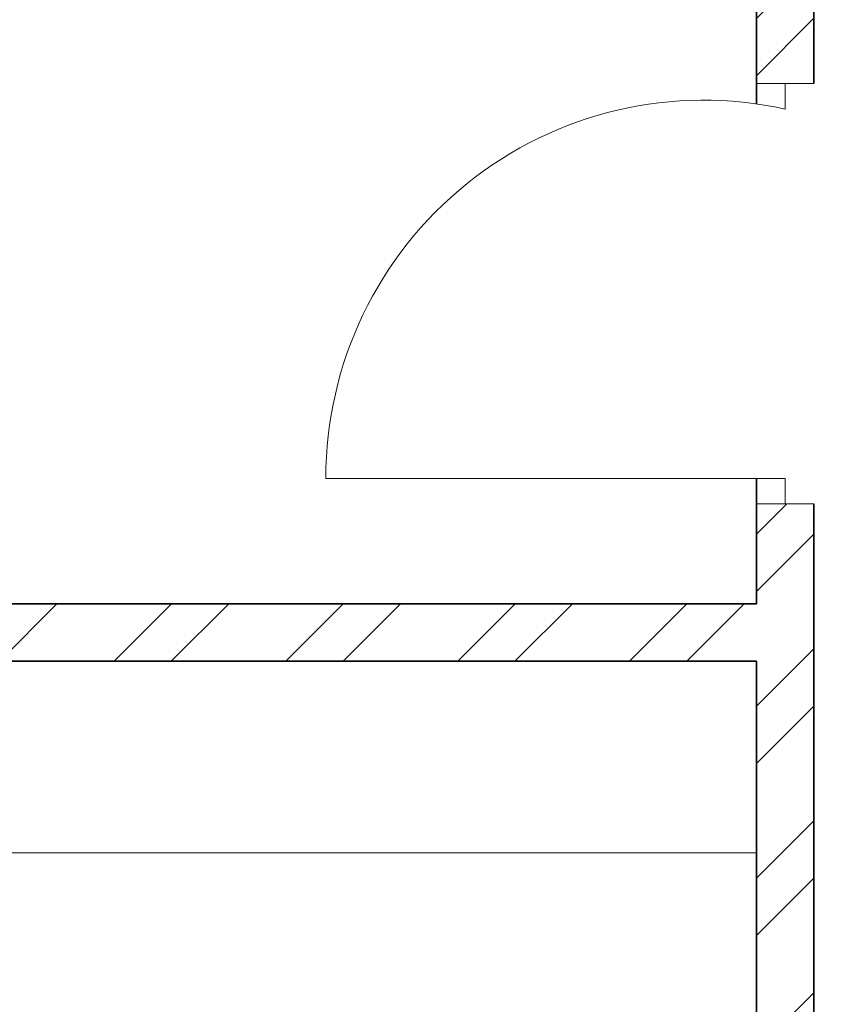
# Model space of a CAD drawing. Units: inches. Extents: x 1962 to 2771, y 1245 to 2660.
# Tile 5 of 114: x 2177 to 2241, y 1753 to 1831. Entities that reach past the tile are written whole.
import ezdxf

# ---------------------------------------------------------------- set-up
doc = ezdxf.new("R2010")
doc.units = ezdxf.units.IN
for name, color, linetype, lineweight in [('A-DOOR', 3, 'Continuous', 18), ('A-FLOR-CASE', 8, 'Continuous', 18), ('A-WALL', 7, 'Continuous', 35), ('A-WALL-PATT', 252, 'Continuous', 13)]:
    doc.layers.add(name, color=color, linetype=linetype, lineweight=lineweight)

msp = doc.modelspace()

# ---------------------------------------------------------------- hatches: boundary and pattern name
at = {"layer": 'A-WALL-PATT'}
h = msp.add_hatch(dxfattribs=at)
h.set_pattern_fill('ANSI32', color=256)
h.paths.add_polyline_path([(2090.8074, 2467.3437), (2141.6481, 2467.3437), (2141.6481, 2469.5937), (2141.6481, 2471.8437), (2086.3074, 2471.8437), (2086.3074, 2422.5333), (2090.8074, 2422.5333)])
h.paths.add_polyline_path([(2282.7664, 2471.8437), (2204.8982, 2471.8437), (2204.8982, 2467.3437), (2234.8074, 2467.3437), (2234.8074, 2311.3437), (2228.7492, 2311.3437), (2228.7492, 2306.8437), (2234.8074, 2306.8437), (2331.9227, 2306.8437), (2331.9227, 2309.0937), (2331.9227, 2311.3437), (2239.3074, 2311.3437), (2239.3074, 2467.3437), (2282.7664, 2467.3437), (2282.7664, 2469.5937)])
h.paths.add_polyline_path([(2471.4531, 2519.8437), (2552.011, 2519.8437), (2564.3996, 2519.8437), (2564.3996, 2511.1389), (2568.8996, 2511.1389), (2568.8996, 2524.3437), (2466.9531, 2524.3437), (2466.9531, 2471.8437), (2450.0749, 2471.8437), (2446.4672, 2471.8437), (2446.4672, 2467.3437), (2450.0749, 2467.3437), (2475.9988, 2467.3437), (2475.9988, 2469.5937), (2475.9988, 2471.8437), (2471.4531, 2471.8437)])
h.paths.add_polyline_path([(2575.2231, 2469.5937), (2575.2231, 2471.8437), (2568.8996, 2471.8437), (2568.8996, 2487.1389), (2564.3996, 2487.1389), (2564.3996, 2471.8437), (2556.511, 2471.8437), (2499.2904, 2471.8437), (2499.2904, 2467.3437), (2507.8074, 2467.3437), (2507.8074, 2311.3437), (2414.863, 2311.3437), (2414.863, 2306.8437), (2512.3074, 2306.8437), (2517.0114, 2306.8437), (2517.0114, 2309.0937), (2517.0114, 2311.3437), (2512.3074, 2311.3437), (2512.3074, 2467.3437), (2575.2231, 2467.3437)])
h.paths.add_polyline_path([(2660.8074, 2471.8437), (2600.9602, 2471.8437), (2600.9602, 2467.3437), (2656.3074, 2467.3437), (2656.3074, 2432.5704), (2660.8074, 2432.5704)])
h.paths.add_polyline_path([(2660.8074, 2372.5704), (2656.3074, 2372.5704), (2656.3074, 2311.3437), (2600.276, 2311.3437), (2600.276, 2309.0937), (2600.276, 2306.8437), (2656.3074, 2306.8437), (2656.3074, 2296.2593), (2660.8074, 2296.2593)])
h.paths.add_polyline_path([(2572.3074, 2306.8437), (2577.1385, 2306.8437), (2577.1385, 2311.3437), (2551.082, 2311.3437), (2551.082, 2306.8437), (2567.8074, 2306.8437), (2567.8074, 2258.8437), (2540.0574, 2258.8437), (2540.0574, 2256.5937), (2540.0574, 2254.3437), (2567.8074, 2254.3437), (2656.3074, 2254.3437), (2656.3074, 2236.9085), (2660.8074, 2236.9085), (2660.8074, 2272.2593), (2656.3074, 2272.2593), (2656.3074, 2258.8437), (2572.3074, 2258.8437)])
h.paths.add_polyline_path([(2512.3074, 2254.3437), (2518.8716, 2254.3437), (2518.8716, 2256.5937), (2518.8716, 2258.8437), (2507.8074, 2258.8437), (2507.8074, 2177.8437), (2567.8074, 2177.8437), (2567.8074, 2172.9628), (2572.3074, 2172.9628), (2572.3074, 2177.8437), (2656.3074, 2177.8437), (2656.3074, 2166.4846), (2660.8074, 2166.4846), (2660.8074, 2200.9085), (2656.3074, 2200.9085), (2656.3074, 2182.3437), (2512.3074, 2182.3437)])
h.paths.add_polyline_path([(2656.3074, 2129.8437), (2572.3074, 2129.8437), (2572.3074, 2150.3044), (2570.0574, 2150.3044), (2567.8074, 2150.3044), (2567.8074, 2129.8437), (2507.8074, 2129.8437), (2507.8074, 2116.3027), (2510.0574, 2116.3027), (2512.3074, 2116.3027), (2512.3074, 2125.3437), (2567.8074, 2125.3437), (2572.3074, 2125.3437), (2656.3074, 2125.3437)])
h.paths.add_polyline_path([(2090.8074, 2362.5333), (2086.3074, 2362.5333), (2086.3074, 2298.6242), (2090.8074, 2298.6242), (2090.8074, 2306.8437), (2174.8074, 2306.8437), (2174.8074, 2286.4178), (2179.3074, 2286.4178), (2179.3074, 2306.8437), (2192.8641, 2306.8437), (2192.8641, 2309.0937), (2192.8641, 2311.3437), (2090.8074, 2311.3437)])
h.paths.add_polyline_path([(2209.156, 2258.8437), (2179.3074, 2258.8437), (2179.3074, 2263.2236), (2177.0574, 2263.2236), (2174.8074, 2263.2236), (2174.8074, 2258.8437), (2090.8074, 2258.8437), (2090.8074, 2274.6242), (2086.3074, 2274.6242), (2086.3074, 2238.2967), (2088.5574, 2238.2967), (2090.8074, 2238.2967), (2090.8074, 2254.3437), (2209.156, 2254.3437)])
h.paths.add_polyline_path([(2090.8074, 2177.8437), (2234.8074, 2177.8437), (2234.8074, 2173.1428), (2239.3074, 2173.1428), (2239.3074, 2258.8437), (2230.8442, 2258.8437), (2230.8442, 2256.5937), (2230.8442, 2254.3437), (2234.8074, 2254.3437), (2234.8074, 2182.3437), (2090.8074, 2182.3437), (2090.8074, 2202.2967), (2086.3074, 2202.2967), (2086.3074, 2140.0389), (2090.8074, 2140.0389)])
h.paths.add_polyline_path([(2090.8074, 2080.0389), (2086.3074, 2080.0389), (2086.3074, 2033.8437), (2090.8074, 2033.8437)], flags=17)
h.paths.add_polyline_path([(2244.9405, 2033.8437), (2239.3074, 2033.8437), (2239.3074, 2142.0665), (2237.2592, 2142.0665), (2234.8074, 2142.0665), (2234.8074, 2033.8437), (2090.8074, 2033.8437), (2076.5204, 2033.8437), (2072.0204, 2033.8437), (2072.0204, 2000.4493), (2076.5204, 2000.4493), (2076.5204, 2029.3437), (2090.8074, 2029.3437), (2244.9405, 2029.3437), (2244.9405, 2031.5937)])
h.paths.add_polyline_path([(2234.8074, 1933.3437), (2076.5204, 1933.3437), (2076.5204, 1952.4493), (2074.2704, 1952.4493), (2072.0204, 1952.4493), (2072.0204, 1933.3437), (2072.0204, 1928.8437), (2234.8074, 1928.8437)])
h.paths.add_polyline_path([(2090.8074, 1928.8437), (2086.3074, 1928.8437), (2086.3074, 1906.5013), (2090.8074, 1906.5013)])
h.paths.add_polyline_path([(2090.8074, 1846.5013), (2086.3074, 1846.5013), (2086.3074, 1769.9917), (2088.5574, 1769.9917), (2090.8074, 1769.9917), (2090.8074, 1780.3437), (2234.8074, 1780.3437), (2234.8074, 1708.3437), (2230.3764, 1708.3437), (2230.3764, 1703.8437), (2239.3074, 1703.8437), (2239.3074, 1792.6669), (2237.0574, 1792.6669), (2234.8074, 1792.6669), (2234.8074, 1784.8437), (2090.8074, 1784.8437)])
h.paths.add_polyline_path([(2239.3074, 1928.8437), (2244.9405, 1928.8437), (2244.9405, 1931.0937), (2244.9405, 1933.3437), (2234.8074, 1933.3437), (2234.8074, 1928.8437), (2234.8074, 1825.5949), (2239.3074, 1825.5949)])
h.paths.add_polyline_path([(2148.0425, 1649.0937), (2148.0425, 1651.3437), (2090.8074, 1651.3437), (2090.8074, 1646.8437), (2148.0425, 1646.8437)], flags=0)
h.paths.add_polyline_path([(2207.5601, 1708.3437), (2090.8074, 1708.3437), (2090.8074, 1703.8437), (2174.8074, 1703.8437), (2174.8074, 1651.3437), (2170.4457, 1651.3437), (2170.4457, 1646.8437), (2195.9924, 1646.8437), (2195.9924, 1649.0937), (2195.9924, 1651.3437), (2179.3074, 1651.3437), (2179.3074, 1703.8437), (2207.5601, 1703.8437), (2207.5601, 1706.0937)])
h.paths.add_polyline_path([(2090.8074, 1733.9917), (2086.3074, 1733.9917), (2086.3074, 1696.1032), (2088.5574, 1696.1032), (2090.8074, 1696.1032)])
h.paths.add_polyline_path([(2090.8074, 1672.1032), (2086.3074, 1672.1032), (2086.3074, 1600.3335), (2090.8074, 1600.3335)])
h.paths.add_polyline_path([(2090.8074, 1540.3335), (2086.3074, 1540.3335), (2086.3074, 1486.3437), (2139.6766, 1486.3437), (2139.6766, 1490.8437), (2090.8074, 1490.8437)])
h.paths.add_polyline_path([(2302.3876, 1490.8437), (2239.3074, 1490.8437), (2239.3074, 1646.8437), (2335.9994, 1646.8437), (2335.9994, 1651.3437), (2229.884, 1651.3437), (2229.884, 1646.8437), (2234.8074, 1646.8437), (2234.8074, 1490.8437), (2202.7103, 1490.8437), (2202.7103, 1488.5937), (2202.7103, 1486.3437), (2275.0699, 1486.3437), (2275.0699, 1475.772), (2279.5699, 1475.772), (2279.5699, 1486.3437), (2302.3876, 1486.3437)])
h.paths.add_polyline_path([(2279.5699, 1451.772), (2275.0699, 1451.772), (2275.0699, 1438.3437), (2174.8074, 1438.3437), (2174.8074, 1486.3437), (2179.7922, 1486.3437), (2179.7922, 1490.8437), (2163.3585, 1490.8437), (2163.3585, 1488.5937), (2163.3585, 1486.3437), (2170.3074, 1486.3437), (2170.3074, 1433.8437), (2279.5699, 1433.8437)])
h.paths.add_polyline_path([(2427.2363, 1490.8437), (2375.8074, 1490.8437), (2375.8074, 1646.8437), (2381.6401, 1646.8437), (2381.6401, 1651.3437), (2365.887, 1651.3437), (2365.887, 1649.0937), (2365.887, 1646.8437), (2371.3074, 1646.8437), (2371.3074, 1490.8437), (2327.5627, 1490.8437), (2327.5627, 1488.5937), (2327.5627, 1486.3437), (2371.3074, 1486.3437), (2371.3074, 1433.8437), (2375.8074, 1433.8437), (2375.8074, 1486.3437), (2427.2363, 1486.3437)])
h.paths.add_polyline_path([(2512.3074, 1646.8437), (2519.4351, 1646.8437), (2519.4351, 1649.0937), (2519.4351, 1651.3437), (2507.8074, 1651.3437), (2416.0063, 1651.3437), (2416.0063, 1649.0937), (2416.0063, 1646.8437), (2507.8074, 1646.8437), (2507.8074, 1490.8437), (2497.0532, 1490.8437), (2497.0532, 1488.5937), (2497.0532, 1486.3437), (2574.9344, 1486.3437), (2574.9344, 1476.0181), (2579.4344, 1476.0181), (2579.4344, 1486.3437), (2584.4872, 1486.3437), (2584.3074, 1490.8437), (2512.3074, 1490.8437)])
h.paths.add_polyline_path([(2470.5091, 1486.3437), (2473.9767, 1486.3437), (2473.9767, 1490.8437), (2449.6605, 1490.8437), (2449.6605, 1488.5937), (2449.6605, 1486.3437), (2466.0091, 1486.3437), (2466.0091, 1433.8437), (2470.5091, 1433.8437), (2579.4344, 1433.8437), (2579.4344, 1452.0181), (2574.9344, 1452.0181), (2574.9344, 1438.3437), (2554.5091, 1438.3437), (2470.5091, 1438.3437)])
h.paths.add_polyline_path([(2656.3074, 1490.8437), (2611.86, 1490.8437), (2611.86, 1486.3437), (2656.3074, 1486.3437)])
h.paths.add_polyline_path([(2660.8074, 1532.7007), (2658.5574, 1532.7007), (2656.3074, 1532.7007), (2656.3074, 1486.3437), (2660.8074, 1486.3437)])
h.paths.add_polyline_path([(2660.8074, 1664.9663), (2656.3074, 1664.9663), (2656.3074, 1651.3437), (2602.2313, 1651.3437), (2602.2313, 1646.8437), (2656.3074, 1646.8437), (2656.3074, 1592.7007), (2660.8074, 1592.7007)])
h.paths.add_polyline_path([(2660.8074, 1724.5221), (2656.3074, 1724.5221), (2656.3074, 1703.8437), (2542.4725, 1703.8437), (2542.4725, 1699.3437), (2567.8074, 1699.3437), (2567.8074, 1651.3437), (2552.7766, 1651.3437), (2552.7766, 1649.0937), (2552.7766, 1646.8437), (2577.2878, 1646.8437), (2577.2878, 1649.0937), (2577.2878, 1651.3437), (2572.3074, 1651.3437), (2572.3074, 1699.3437), (2656.3074, 1699.3437), (2656.3074, 1688.9663), (2660.8074, 1688.9663)])
h.paths.add_polyline_path([(2660.8074, 1880.6524), (2656.3074, 1880.6524), (2656.3074, 1832.8437), (2512.3074, 1832.8437), (2512.3074, 1837.8959), (2507.8074, 1837.8959), (2507.8074, 1828.3437), (2567.8074, 1828.3437), (2567.8074, 1804.3437), (2572.3074, 1804.3437), (2572.3074, 1828.3437), (2656.3074, 1828.3437), (2656.3074, 1818.6778), (2660.8074, 1818.6778)])
h.paths.add_polyline_path([(2660.8074, 1794.6778), (2656.3074, 1794.6778), (2656.3074, 1780.3437), (2572.3074, 1780.3437), (2572.3074, 1783.0303), (2570.0574, 1783.0303), (2567.8074, 1783.0303), (2567.8074, 1780.3437), (2507.8074, 1780.3437), (2507.8074, 1699.3437), (2517.8858, 1699.3437), (2517.8858, 1701.5937), (2517.8858, 1703.8437), (2512.3074, 1703.8437), (2512.3074, 1775.8437), (2656.3074, 1775.8437), (2656.3074, 1760.5221), (2660.8074, 1760.5221)])
h.paths.add_polyline_path([(2660.8074, 1981.3437), (2660.8074, 2020.2808), (2658.5574, 2020.2808), (2656.3074, 2020.2808), (2656.3074, 1981.3437), (2512.3074, 1981.3437), (2512.3074, 2086.6996), (2507.8074, 2086.6996), (2507.8074, 1981.3437), (2375.8074, 1981.3437), (2375.8074, 1986.8505), (2373.5574, 1986.8505), (2371.3074, 1986.8505), (2371.3074, 1973.2607), (2375.8074, 1973.2607), (2375.8074, 1976.8437), (2507.8074, 1976.8437), (2507.8074, 1865.4281), (2510.0574, 1865.4281), (2512.3074, 1865.4281), (2512.3074, 1976.8437), (2660.8074, 1976.8437)])
h.paths.add_polyline_path([(2375.8074, 1940.297), (2373.5574, 1940.297), (2371.3074, 1940.297), (2371.3074, 1933.3437), (2278.4434, 1933.3437), (2278.4434, 1928.8437), (2371.3074, 1928.8437), (2371.3074, 1651.3437), (2375.8074, 1651.3437)])
h.paths.add_polyline_path([(2660.8074, 1976.8437), (2656.3074, 1976.8437), (2656.3074, 1940.6524), (2660.8074, 1940.6524)], flags=17)
h.paths.add_polyline_path([(2660.8074, 2142.4846), (2656.3074, 2142.4846), (2656.3074, 2080.2808), (2660.8074, 2080.2808)])
h.paths.add_polyline_path([(2381.4189, 2311.3437), (2375.8074, 2311.3437), (2375.8074, 2467.3437), (2424.7242, 2467.3437), (2424.7242, 2469.5937), (2424.7242, 2471.8437), (2375.8074, 2471.8437), (2375.8074, 2524.3437), (2371.3074, 2524.3437), (2371.3074, 2471.8437), (2307.2097, 2471.8437), (2307.2097, 2467.3437), (2371.3074, 2467.3437), (2371.3074, 2311.3437), (2366.8901, 2311.3437), (2366.8901, 2306.8437), (2371.3074, 2306.8437), (2371.3074, 2033.8437), (2279.6589, 2033.8437), (2279.6589, 2029.3437), (2371.3074, 2029.3437), (2371.3074, 2014.2598), (2375.8074, 2014.2598), (2375.8074, 2306.8437), (2381.4189, 2306.8437)])
h.paths.add_polyline_path([(2263.3074, 2524.3437), (2170.3074, 2524.3437), (2170.3074, 2519.8437), (2170.3074, 2471.8437), (2165.0312, 2471.8437), (2165.0312, 2467.3437), (2179.6721, 2467.3437), (2179.6721, 2469.5161), (2179.6721, 2471.8437), (2174.8074, 2471.8437), (2174.8074, 2519.8437), (2258.8074, 2519.8437), (2258.8074, 2511.6436), (2263.3074, 2511.6436)])
h.paths.add_polyline_path([(2245.0232, 1361.4123), (2492.9468, 1361.4123), (2492.9468, 1398.505), (2245.0232, 1398.505)], flags=9)
h.paths.add_polyline_path([(2388.1434, 2086.6936), (2425.0704, 2086.6936), (2425.0704, 2105.3509), (2388.1434, 2105.3509)], flags=9)
h.paths.add_polyline_path([(2404.922, 2242.6744), (2445.7337, 2242.6744), (2445.7337, 2261.3318), (2404.922, 2261.3318)], flags=9)
h.paths.add_polyline_path([(2269.4107, 2156.7935), (2306.3378, 2156.7935), (2306.3378, 2175.4508), (2269.4107, 2175.4508)], flags=9)
h.paths.add_polyline_path([(2269.3277, 2233.4343), (2306.2547, 2233.4343), (2306.2547, 2252.0917), (2269.3277, 2252.0917)], flags=9)
h.paths.add_polyline_path([(2431.6052, 2320.6922), (2470.4456, 2320.6922), (2470.4456, 2339.3495), (2431.6052, 2339.3495)], flags=25)
h.paths.add_polyline_path([(2249.6902, 2315.7608), (2288.5306, 2315.7608), (2288.5306, 2334.4182), (2249.6902, 2334.4182)], flags=25)
h.paths.add_polyline_path([(2096.9301, 2314.3181), (2135.7704, 2314.3181), (2135.7704, 2332.9755), (2096.9301, 2332.9755)], flags=25)
h.paths.add_polyline_path([(2134.3475, 2285.7089), (2161.4655, 2285.7089), (2161.4655, 2304.3662), (2134.3475, 2304.3662)], flags=9)
h.paths.add_polyline_path([(2126.5155, 2209.4076), (2159.9227, 2209.4076), (2159.9227, 2228.065), (2126.5155, 2228.065)], flags=25)
h.paths.add_polyline_path([(2110.5753, 2141.5299), (2149.4157, 2141.5299), (2149.4157, 2160.1872), (2110.5753, 2160.1872)], flags=25)
h.paths.add_polyline_path([(2249.8618, 1968.3317), (2286.3966, 1968.3317), (2286.3966, 1986.989), (2249.8618, 1986.989)], flags=9)
h.paths.add_polyline_path([(2395.9507, 1777.0051), (2436.7624, 1777.0051), (2436.7624, 1795.6625), (2395.9507, 1795.6625)], flags=9)
h.paths.add_polyline_path([(2398.5259, 1888.5651), (2435.0062, 1888.5651), (2435.0062, 1907.2224), (2398.5259, 1907.2224)], flags=25)
h.paths.add_polyline_path([(2259.3506, 1728.3559), (2296.2776, 1728.3559), (2296.2776, 1747.0132), (2259.3506, 1747.0132)], flags=9)
h.paths.add_polyline_path([(2271.3698, 1845.268), (2308.2968, 1845.268), (2308.2968, 1863.9253), (2271.3698, 1863.9253)], flags=9)
h.paths.add_polyline_path([(2120.9355, 1786.3027), (2159.7759, 1786.3027), (2159.7759, 1804.9601), (2120.9355, 1804.9601)], flags=25)
h.paths.add_polyline_path([(2121.3164, 1732.1043), (2154.7236, 1732.1043), (2154.7236, 1750.7616), (2121.3164, 1750.7616)], flags=25)
h.paths.add_polyline_path([(2118.3706, 1678.8997), (2147.5282, 1678.8997), (2147.5282, 1697.557), (2118.3706, 1697.557)], flags=25)
h.paths.add_polyline_path([(2385.9227, 1493.557), (2424.763, 1493.557), (2424.763, 1512.2143), (2385.9227, 1512.2143)], flags=25)
h.paths.add_polyline_path([(2248.7058, 1500.0256), (2287.5462, 1500.0256), (2287.5462, 1518.6829), (2248.7058, 1518.6829)], flags=25)
h.paths.add_polyline_path([(2104.1669, 1617.3771), (2143.0073, 1617.3771), (2143.0073, 1636.0344), (2104.1669, 1636.0344)], flags=9)
h.paths.add_polyline_path([(2096.0714, 1447.8824), (2137.3845, 1447.8824), (2137.3845, 1458.1859), (2096.0714, 1458.1859)], flags=9)
h.paths.add_polyline_path([(2180.6114, 1440.325), (2209.7689, 1440.325), (2209.7689, 1458.9823), (2180.6114, 1458.9823)], flags=25)
h.paths.add_polyline_path([(2316.1698, 1447.9637), (2357.4829, 1447.9637), (2357.4829, 1458.2673), (2316.1698, 1458.2673)], flags=9)
h.paths.add_polyline_path([(2397.6187, 1447.9637), (2438.9318, 1447.9637), (2438.9318, 1458.2673), (2397.6187, 1458.2673)], flags=9)
h.paths.add_polyline_path([(2473.0778, 1439.5953), (2502.2354, 1439.5953), (2502.2354, 1458.2527), (2473.0778, 1458.2527)], flags=25)
h.paths.add_polyline_path([(2589.7027, 1447.8819), (2631.0158, 1447.8819), (2631.0158, 1458.1855), (2589.7027, 1458.1855)], flags=9)
h.paths.add_polyline_path([(2522.4009, 1497.5285), (2561.2413, 1497.5285), (2561.2413, 1516.1859), (2522.4009, 1516.1859)], flags=25)
h.paths.add_polyline_path([(2579.6565, 1671.3482), (2608.8141, 1671.3482), (2608.8141, 1690.0056), (2579.6565, 1690.0056)], flags=25)
h.paths.add_polyline_path([(2544.7038, 1725.5064), (2578.1111, 1725.5064), (2578.1111, 1744.1637), (2544.7038, 1744.1637)], flags=25)
h.paths.add_polyline_path([(2578.1191, 1807.472), (2607.2766, 1807.472), (2607.2766, 1826.1293), (2578.1191, 1826.1293)], flags=25)
h.paths.add_polyline_path([(2595.0614, 1835.1839), (2633.9018, 1835.1839), (2633.9018, 1853.8413), (2595.0614, 1853.8413)], flags=25)
h.paths.add_polyline_path([(2567.0097, 2097.7035), (2605.8501, 2097.7035), (2605.8501, 2116.3609), (2567.0097, 2116.3609)], flags=9)
h.paths.add_polyline_path([(2586.644, 2134.6454), (2615.8015, 2134.6454), (2615.8015, 2153.3027), (2586.644, 2153.3027)], flags=9)
h.paths.add_polyline_path([(2544.6185, 2212.6783), (2578.0258, 2212.6783), (2578.0258, 2231.3356), (2544.6185, 2231.3356)], flags=25)
h.paths.add_polyline_path([(2577.0273, 2256.9023), (2606.1849, 2256.9023), (2606.1849, 2275.5597), (2577.0273, 2275.5597)], flags=24)
h.paths.add_polyline_path([(2605.2683, 2315.2821), (2644.1087, 2315.2821), (2644.1087, 2333.9395), (2605.2683, 2333.9395)], flags=25)
h.paths.add_polyline_path([(2583.1244, 2496.1815), (2624.4375, 2496.1815), (2624.4375, 2506.4851), (2583.1244, 2506.4851)], flags=9)
h.paths.add_polyline_path([(2474.761, 2497.0823), (2503.9185, 2497.0823), (2503.9185, 2515.7397), (2474.761, 2515.7397)], flags=25)
h.paths.add_polyline_path([(2387.5787, 2494.2563), (2428.902, 2494.2563), (2428.902, 2504.5598), (2387.5787, 2504.5598)], flags=9)
h.paths.add_polyline_path([(2300.1657, 2500.1564), (2341.4788, 2500.1564), (2341.4788, 2510.46), (2300.1657, 2510.46)], flags=25)
h.paths.add_polyline_path([(2176.8589, 2497.5843), (2206.0165, 2497.5843), (2206.0165, 2516.2416), (2176.8589, 2516.2416)], flags=25)
h.paths.add_polyline_path([(2097.4668, 2494.9762), (2138.7799, 2494.9762), (2138.7799, 2505.2798), (2097.4668, 2505.2798)], flags=9)

# ---------------------------------------------------------------- linework, layer by layer
at = {"layer": 'A-DOOR'}
for p, q in [((2234.8074, 1825.5949), (2239.3074, 1825.5949)), ((2239.3074, 1825.5949), (2237.0574, 1825.5949)), ((2237.0574, 1825.5949), (2237.0574, 1823.5949)), ((2237.0574, 1794.6669), (2201.0574, 1794.6669)), ((2237.0574, 1792.6669), (2237.0574, 1794.6669)), ((2234.8074, 1792.6669), (2239.3074, 1792.6669)), ((2239.3074, 1792.6669), (2237.0574, 1792.6669))]:
    msp.add_line(p, q, dxfattribs=at)
msp.add_arc((2230.6801, 1794.6669), 29.6227, 77.567746, 180, dxfattribs=at)
at = {"layer": 'A-FLOR-CASE'}
msp.add_line((2110.6655, 1765.3193), (2234.8074, 1765.3193), dxfattribs=at)
at = {"layer": 'A-WALL'}
for p, q in [((2234.8074, 1933.3437), (2234.8074, 1824.0006)), ((2239.3074, 1928.8437), (2239.3074, 1825.5949)), ((2234.8074, 1794.6669), (2234.8074, 1784.8437)), ((2239.3074, 1792.6669), (2239.3074, 1703.8437)), ((2090.8074, 1784.8437), (2234.8074, 1784.8437)), ((2090.8074, 1780.3437), (2234.8074, 1780.3437)), ((2234.8074, 1780.3437), (2234.8074, 1708.3437))]:
    msp.add_line(p, q, dxfattribs=at)

doc.saveas('drawing.dxf')
